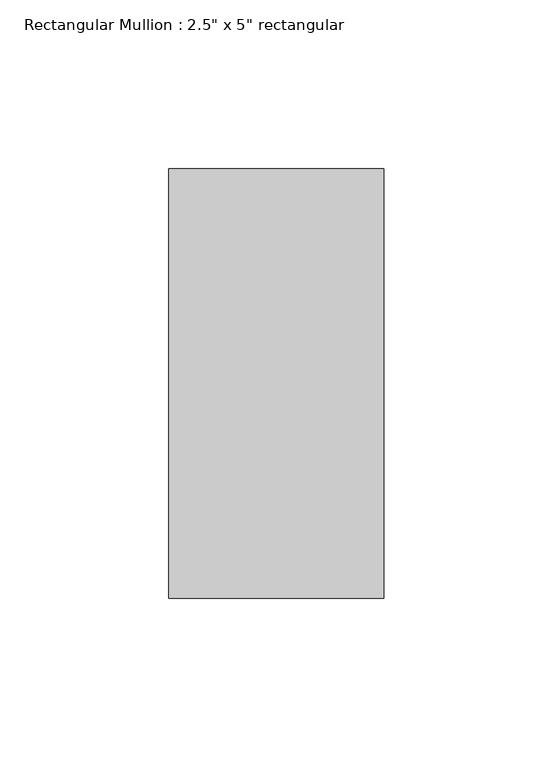
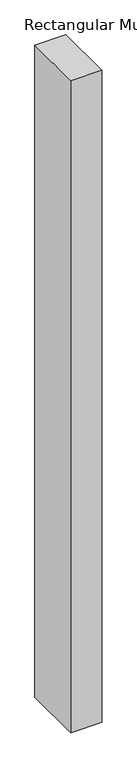
"""IFC4 building model written with IfcOpenShell, lengths in millimetres: member geometry."""

from ifc_helpers import new_model, si_unit, frame, origin, place, context, project, spatial, polyline, outline, extrude, source, transform, mapped, element, save


def member_d44a35f4(model_context):
    return source(origin(), model_context, "Body", "SweptSolid", [
        extrude(outline(polyline([(31.75, 63.5), (31.75, -63.5), (-31.75, -63.5), (-31.75, 63.5), (31.75, 63.5)])), frame((0.0, 0.0, -1411.7908292), z_axis=(0.0, 0.0, 1.0), x_axis=(1.0, 0.0, 0.0)), (0.0, 0.0, 1.0), 1411.7908292),
    ])


if __name__ == "__main__":
    model = new_model("IFC4")
    model_context = context("Model", 3, world=origin())
    ifc_project = project(units=[si_unit("LENGTHUNIT", "METRE", prefix="MILLI")], contexts=[model_context])
    site = spatial("IfcSite", under=ifc_project)
    building = spatial("IfcBuilding", under=site)
    placement = place(None, origin())
    member_shape = member_d44a35f4(model_context)
    element("IfcMember", 1, ObjectType="Rectangular Mullion : 2.5\" x 5\" rectangular", at=placement, inside=building, context=model_context, shape_type="MappedRepresentation", body=[
        mapped(member_shape, transform((0.0, 0.0, 0.0), x_axis=(1.0, 0.0, 0.0), y_axis=(0.0, 1.0, 0.0), z_axis=(0.0, 0.0, 1.0))),
    ])
    save(model, "model.ifc")

# Revit data of these elements
# Type "Rectangular Mullion : 2.5\" x 5\" rectangular"
#   built-in parameter 1007304 = 0.416667 (stored number, unit not read)
#   built-in parameter 1007301 = 0.104167 (stored number, unit not read)
#   built-in parameter 1007300 = 0.104167 (stored number, unit not read)
# Element 1 (IfcMember, "Rectangular Mullion : 2.5\" x 5\" rectangular")
#   Materials on its faces: "Aluminum"
# Materials
#   "Aluminum": class "Metal", colour RGB 247 247 247, transparency 0, Description = "Aluminum 6061", Cost = 0
